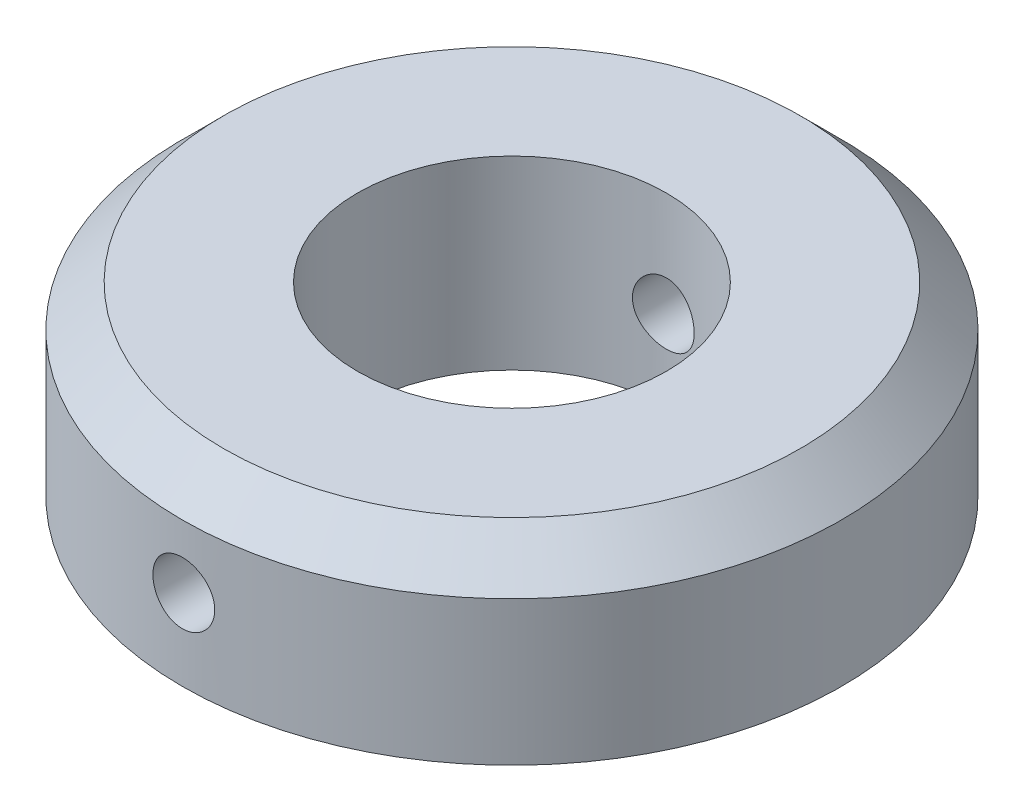
ISO-10303-21;
HEADER;
FILE_DESCRIPTION(('STEP AP214'),'2;1');
FILE_NAME('part.step','',(''),(''),'','','');
FILE_SCHEMA(('AUTOMOTIVE_DESIGN { 1 0 10303 214 1 1 1 1 }'));
ENDSEC;
DATA;
#1=APPLICATION_CONTEXT('core data for automotive mechanical design processes');
#2=APPLICATION_PROTOCOL_DEFINITION('international standard','automotive_design',2000,#1);
#3=PRODUCT_CONTEXT('',#1,'mechanical');
#4=PRODUCT('Part','Part','',(#3));
#5=PRODUCT_RELATED_PRODUCT_CATEGORY('part','',(#4));
#6=PRODUCT_DEFINITION_FORMATION('','',#4);
#7=PRODUCT_DEFINITION_CONTEXT('part definition',#1,'design');
#8=PRODUCT_DEFINITION('design','',#6,#7);
#9=PRODUCT_DEFINITION_SHAPE('','',#8);
#10=(LENGTH_UNIT() NAMED_UNIT(*) SI_UNIT(.MILLI.,.METRE.));
#11=(NAMED_UNIT(*) PLANE_ANGLE_UNIT() SI_UNIT($,.RADIAN.));
#12=(NAMED_UNIT(*) SI_UNIT($,.STERADIAN.) SOLID_ANGLE_UNIT());
#13=UNCERTAINTY_MEASURE_WITH_UNIT(LENGTH_MEASURE(1.E-05),#10,'distance_accuracy_value','');
#14=(GEOMETRIC_REPRESENTATION_CONTEXT(3) GLOBAL_UNCERTAINTY_ASSIGNED_CONTEXT((#13)) GLOBAL_UNIT_ASSIGNED_CONTEXT((#10,
#11,#12)) REPRESENTATION_CONTEXT('',''));
#15=CARTESIAN_POINT('',(0.,0.,0.));
#16=DIRECTION('',(0.,0.,1.));
#17=DIRECTION('',(1.,0.,0.));
#18=AXIS2_PLACEMENT_3D('',#15,#16,#17);
#19=CARTESIAN_POINT('',(0.,9.,0.));
#20=DIRECTION('',(0.,1.,0.));
#21=DIRECTION('',(0.,0.,1.));
#22=AXIS2_PLACEMENT_3D('',#19,#20,#21);
#23=PLANE('',#22);
#24=CARTESIAN_POINT('',(0.,9.,0.));
#25=DIRECTION('',(0.,1.,0.));
#26=DIRECTION('',(0.,0.,1.));
#27=AXIS2_PLACEMENT_3D('',#24,#25,#26);
#28=CIRCLE('',#27,14.);
#29=CARTESIAN_POINT('',(0.,9.,14.));
#30=VERTEX_POINT('',#29);
#31=EDGE_CURVE('E52',#30,#30,#28,.T.);
#32=ORIENTED_EDGE('',*,*,#31,.T.);
#33=EDGE_LOOP('',(#32));
#34=FACE_BOUND('',#33,.T.);
#35=CARTESIAN_POINT('',(0.,9.,0.));
#36=DIRECTION('',(0.,1.,0.));
#37=DIRECTION('',(0.,0.,1.));
#38=AXIS2_PLACEMENT_3D('',#35,#36,#37);
#39=CIRCLE('',#38,7.5);
#40=CARTESIAN_POINT('',(0.,9.,7.5));
#41=VERTEX_POINT('',#40);
#42=EDGE_CURVE('E110',#41,#41,#39,.T.);
#43=ORIENTED_EDGE('',*,*,#42,.F.);
#44=EDGE_LOOP('',(#43));
#45=FACE_BOUND('',#44,.T.);
#46=ADVANCED_FACE('F39',(#34,#45),#23,.T.);
#47=CARTESIAN_POINT('',(0.,0.,0.));
#48=DIRECTION('',(0.,1.,0.));
#49=DIRECTION('',(0.,0.,1.));
#50=AXIS2_PLACEMENT_3D('',#47,#48,#49);
#51=PLANE('',#50);
#52=CARTESIAN_POINT('',(0.,0.,0.));
#53=DIRECTION('',(0.,1.,0.));
#54=DIRECTION('',(0.,0.,1.));
#55=AXIS2_PLACEMENT_3D('',#52,#53,#54);
#56=CIRCLE('',#55,16.);
#57=CARTESIAN_POINT('',(0.,0.,16.));
#58=VERTEX_POINT('',#57);
#59=EDGE_CURVE('E59',#58,#58,#56,.T.);
#60=ORIENTED_EDGE('',*,*,#59,.F.);
#61=EDGE_LOOP('',(#60));
#62=FACE_BOUND('',#61,.T.);
#63=CARTESIAN_POINT('',(0.,0.,0.));
#64=DIRECTION('',(0.,1.,0.));
#65=DIRECTION('',(0.,0.,1.));
#66=AXIS2_PLACEMENT_3D('',#63,#64,#65);
#67=CIRCLE('',#66,7.5);
#68=CARTESIAN_POINT('',(0.,0.,7.5));
#69=VERTEX_POINT('',#68);
#70=EDGE_CURVE('E108',#69,#69,#67,.T.);
#71=ORIENTED_EDGE('',*,*,#70,.T.);
#72=EDGE_LOOP('',(#71));
#73=FACE_BOUND('',#72,.T.);
#74=ADVANCED_FACE('F91',(#62,#73),#51,.F.);
#75=CARTESIAN_POINT('',(0.,9.,0.));
#76=DIRECTION('',(0.,-1.,0.));
#77=DIRECTION('',(0.,0.,-1.));
#78=AXIS2_PLACEMENT_3D('',#75,#76,#77);
#79=CYLINDRICAL_SURFACE('',#78,16.);
#80=CARTESIAN_POINT('',(0.,5.43034536282499,-16.));
#81=CARTESIAN_POINT('',(-0.0840576996574437,5.43034170985044,-15.9999990874377));
#82=CARTESIAN_POINT('',(-0.168171627589379,5.423255885696,-15.9993305431474));
#83=CARTESIAN_POINT('',(-0.334069380755584,5.39509506295832,-15.9967278705616));
#84=CARTESIAN_POINT('',(-0.41585050405935,5.37400447917629,-15.9947923323258));
#85=CARTESIAN_POINT('',(-0.574656127608676,5.31845188267265,-15.9898742536092));
#86=CARTESIAN_POINT('',(-0.65168339804474,5.28399774416038,-15.9868923297887));
#87=CARTESIAN_POINT('',(-0.798844080486045,5.20271088579991,-15.9802152971296));
#88=CARTESIAN_POINT('',(-0.868978900331676,5.15588070110172,-15.9765203343939));
#89=CARTESIAN_POINT('',(-1.00060451358299,5.05101076457032,-15.9688182603974));
#90=CARTESIAN_POINT('',(-1.06207030524923,4.99293969202882,-15.9648102960756));
#91=CARTESIAN_POINT('',(-1.17439832001845,4.86730300549484,-15.9569410358395));
#92=CARTESIAN_POINT('',(-1.22526006263066,4.79973696149825,-15.9530797465779));
#93=CARTESIAN_POINT('',(-1.31502335742932,4.6568736146017,-15.9459321531903));
#94=CARTESIAN_POINT('',(-1.3539025185592,4.58156218431094,-15.9426469303983));
#95=CARTESIAN_POINT('',(-1.41845402355083,4.42544403169777,-15.9370337331836));
#96=CARTESIAN_POINT('',(-1.44412665669788,4.34463742978944,-15.9347057377932));
#97=CARTESIAN_POINT('',(-1.48146280171703,4.18007617451122,-15.9312781055131));
#98=CARTESIAN_POINT('',(-1.4931675262139,4.09633094808939,-15.9301748556596));
#99=CARTESIAN_POINT('',(-1.50236296529023,3.92805789753474,-15.9293103424401));
#100=CARTESIAN_POINT('',(-1.49985401107328,3.84353009168322,-15.9295490478042));
#101=CARTESIAN_POINT('',(-1.48072731632193,3.67637474710345,-15.9313381803757));
#102=CARTESIAN_POINT('',(-1.46415449112824,3.59374201798684,-15.9328844316596));
#103=CARTESIAN_POINT('',(-1.41744034122964,3.43243614206901,-15.9371079001961));
#104=CARTESIAN_POINT('',(-1.3872988532664,3.35376304292278,-15.9397851310565));
#105=CARTESIAN_POINT('',(-1.3142531244971,3.20246728495301,-15.9459737103685));
#106=CARTESIAN_POINT('',(-1.27132886758545,3.12985434553073,-15.9494863652322));
#107=CARTESIAN_POINT('',(-1.17395046357292,2.9928464513137,-15.9569488633928));
#108=CARTESIAN_POINT('',(-1.11949602014408,2.92845170779631,-15.9608987179246));
#109=CARTESIAN_POINT('',(-1.0003517239972,2.80944707192839,-15.9688091656293));
#110=CARTESIAN_POINT('',(-0.935623065481643,2.7548760222016,-15.9727697411833));
#111=CARTESIAN_POINT('',(-0.797902747560453,2.65736861347273,-15.980240887844));
#112=CARTESIAN_POINT('',(-0.724911080506018,2.61443226524064,-15.9837514585342));
#113=CARTESIAN_POINT('',(-0.572710457840157,2.54141496340302,-15.9899280035071));
#114=CARTESIAN_POINT('',(-0.493500599071182,2.51133588134771,-15.9925938548147));
#115=CARTESIAN_POINT('',(-0.331124322273424,2.46491490921607,-15.9967792828423));
#116=CARTESIAN_POINT('',(-0.247958008264099,2.44857265819436,-15.9982988896806));
#117=CARTESIAN_POINT('',(-0.0803661051891792,2.43013829263682,-16.0000167439267));
#118=CARTESIAN_POINT('',(0.00405353705355389,2.42799255769071,-16.0002199632847));
#119=CARTESIAN_POINT('',(0.17205127843741,2.43787144609971,-15.9992954563897));
#120=CARTESIAN_POINT('',(0.25562938753764,2.44989590155872,-15.9981677459063));
#121=CARTESIAN_POINT('',(0.419417565662278,2.48772937270583,-15.9947113308173));
#122=CARTESIAN_POINT('',(0.499633460781156,2.51351338202034,-15.9923848051808));
#123=CARTESIAN_POINT('',(0.654601026064808,2.57810841177009,-15.9867919001555));
#124=CARTESIAN_POINT('',(0.729352587838971,2.61691969052914,-15.9835255021299));
#125=CARTESIAN_POINT('',(0.871512627170616,2.70660122899258,-15.9764061412804));
#126=CARTESIAN_POINT('',(0.938898720136997,2.75750683429548,-15.9725514712721));
#127=CARTESIAN_POINT('',(1.06418863953514,2.86988117350934,-15.9646938863657));
#128=CARTESIAN_POINT('',(1.12209225711382,2.93135014001898,-15.9606909682048));
#129=CARTESIAN_POINT('',(1.22695884240091,3.06333978161952,-15.9529731744665));
#130=CARTESIAN_POINT('',(1.27388669789138,3.13388841685224,-15.9492592480101));
#131=CARTESIAN_POINT('',(1.35522852111172,3.28189637233934,-15.9425540145368));
#132=CARTESIAN_POINT('',(1.38964264189423,3.35935560805731,-15.9395626986821));
#133=CARTESIAN_POINT('',(1.44492091464444,3.51886401781301,-15.9346470864828));
#134=CARTESIAN_POINT('',(1.46580619653949,3.60090581582139,-15.9327211269093));
#135=CARTESIAN_POINT('',(1.49350258954047,3.76735064147414,-15.9301489811257));
#136=CARTESIAN_POINT('',(1.50031405119065,3.8517536102545,-15.9295027630406));
#137=CARTESIAN_POINT('',(1.49966491440228,4.02017592399092,-15.929563861851));
#138=CARTESIAN_POINT('',(1.49225947642594,4.1041954889146,-15.930265947437));
#139=CARTESIAN_POINT('',(1.46350215815381,4.26979160292843,-15.9329334080922));
#140=CARTESIAN_POINT('',(1.44215025977346,4.35136814885054,-15.9348987847997));
#141=CARTESIAN_POINT('',(1.38612086380733,4.50976370527025,-15.9398699587172));
#142=CARTESIAN_POINT('',(1.35144474478351,4.5865832069908,-15.9428756482903));
#143=CARTESIAN_POINT('',(1.26975707915473,4.73331997686405,-15.9495889947787));
#144=CARTESIAN_POINT('',(1.22274565072801,4.80323731113401,-15.9532966449687));
#145=CARTESIAN_POINT('',(1.1175144922873,4.93446768251109,-15.9610133498176));
#146=CARTESIAN_POINT('',(1.05925372920377,4.99574775354154,-15.9650234741094));
#147=CARTESIAN_POINT('',(0.933256833294973,5.10768719699359,-15.97288349636));
#148=CARTESIAN_POINT('',(0.865518425328446,5.15834401194823,-15.9767333555577));
#149=CARTESIAN_POINT('',(0.722325032343342,5.24768622001424,-15.9838478838907));
#150=CARTESIAN_POINT('',(0.646852995234792,5.28634436712216,-15.9871112141985));
#151=CARTESIAN_POINT('',(0.490507906890444,5.35038854209055,-15.9926700583075));
#152=CARTESIAN_POINT('',(0.409641110987895,5.37578965014847,-15.9949666711945));
#153=CARTESIAN_POINT('',(0.273590626043441,5.40621111478394,-15.997751278192));
#154=CARTESIAN_POINT('',(0.219278798513779,5.41524922609769,-15.9985906537126));
#155=CARTESIAN_POINT('',(0.109986004796567,5.42731753475249,-15.9997153122197));
#156=CARTESIAN_POINT('',(0.0550050409638892,5.43034775323081,-16.0000005971556));
#157=CARTESIAN_POINT('',(0.,5.43034536282499,-16.));
#158=B_SPLINE_CURVE_WITH_KNOTS('',3,(#80,#81,#82,#83,#84,#85,#86,#87,#88,#89,#90,#91,#92,#93,
#94,#95,#96,#97,#98,#99,#100,#101,#102,#103,#104,#105,#106,#107,#108,#109,#110,#111,#112,#113,
#114,#115,#116,#117,#118,#119,#120,#121,#122,#123,#124,#125,#126,#127,#128,#129,#130,#131,#132,
#133,#134,#135,#136,#137,#138,#139,#140,#141,#142,#143,#144,#145,#146,#147,#148,#149,#150,#151,
#152,#153,#154,#155,#156,#157),.UNSPECIFIED.,.T.,.F.,(4,2,2,2,2,2,2,2,2,2,2,2,2,2,2,2,2,2,2,2,2,
2,2,2,2,2,2,2,2,2,2,2,2,2,2,2,2,2,4),(0.,0.251972252870636,0.504225384091021,0.756330105411321,
1.00838322474624,1.26114902549997,1.51392627709208,1.7671730523228,2.02041428001784,
2.27290645171288,2.52539273992279,2.77707569221288,3.02876167283653,3.28084385105098,
3.53293250861135,3.78599701442565,4.03906175449559,4.29216331905139,4.54525823296866,
4.79739665595728,5.04953209150326,5.30121085328536,5.55289460601788,5.80532315252837,
6.05775725807137,6.31098819719604,6.56421603900671,6.81704741885484,7.06987250121943,
7.32171862414045,7.57356507363443,7.82538547338789,8.07720346066821,8.32995794997956,
8.58277321830877,8.8361584370252,9.08925479233284,9.25413906717824,9.41902276191882),.UNSPECIFIED.);
#159=CARTESIAN_POINT('',(0.,5.43034536282499,-16.));
#160=VERTEX_POINT('',#159);
#161=EDGE_CURVE('E85',#160,#160,#158,.T.);
#162=ORIENTED_EDGE('',*,*,#161,.T.);
#163=EDGE_LOOP('',(#162));
#164=FACE_BOUND('',#163,.T.);
#165=CARTESIAN_POINT('',(1.5,3.93034536282499,15.929532322074));
#166=CARTESIAN_POINT('',(1.49999634620447,3.84628857842711,15.9295332496796));
#167=CARTESIAN_POINT('',(1.49291067114191,3.76217556284008,15.9302048142922));
#168=CARTESIAN_POINT('',(1.46475049444749,3.59627970529378,15.9328182764505));
#169=CARTESIAN_POINT('',(1.44366040446064,3.51449956598149,15.9347615895481));
#170=CARTESIAN_POINT('',(1.38810925248868,3.3556960230131,15.9396965331442));
#171=CARTESIAN_POINT('',(1.35365608820284,3.27866984083425,15.9426875443425));
#172=CARTESIAN_POINT('',(1.27237152401549,3.13151098150667,15.9493801055301));
#173=CARTESIAN_POINT('',(1.22554265686883,3.06137689787688,15.9530815100911));
#174=CARTESIAN_POINT('',(1.12067405070444,2.92975045195916,15.9607911339043));
#175=CARTESIAN_POINT('',(1.062602696675,2.86828332491989,15.9648001986727));
#176=CARTESIAN_POINT('',(0.936964886657167,2.75595273324473,15.9726657227971));
#177=CARTESIAN_POINT('',(0.869398004306441,2.70508974500413,15.9765221752908));
#178=CARTESIAN_POINT('',(0.726533924195945,2.6153251486955,15.9836561919841));
#179=CARTESIAN_POINT('',(0.651222743202337,2.57644570262144,15.9869326789076));
#180=CARTESIAN_POINT('',(0.495105132470078,2.5118936020372,15.9925284235434));
#181=CARTESIAN_POINT('',(0.414298821735456,2.48622066162639,15.9948477019775));
#182=CARTESIAN_POINT('',(0.249738452457438,2.44888387300111,15.9982617839516));
#183=CARTESIAN_POINT('',(0.165993826496405,2.43717878581782,15.9993601913537));
#184=CARTESIAN_POINT('',(-0.00227804877261734,2.42798241333139,16.0002210112843));
#185=CARTESIAN_POINT('',(-0.0868052800149707,2.43049080073753,15.9999834545757));
#186=CARTESIAN_POINT('',(-0.253963127789742,2.44961659939017,15.9982020712559));
#187=CARTESIAN_POINT('',(-0.336598868002988,2.46618966582899,15.9966623503171));
#188=CARTESIAN_POINT('',(-0.497910641604227,2.51290534244825,15.9924544533603));
#189=CARTESIAN_POINT('',(-0.57658662892854,2.54304811044404,15.9897862642183));
#190=CARTESIAN_POINT('',(-0.727885882948087,2.61609648693961,15.9836144229149));
#191=CARTESIAN_POINT('',(-0.80049957541682,2.65902181244727,15.9801094817377));
#192=CARTESIAN_POINT('',(-0.937508522273802,2.75640249573777,15.9726576575237));
#193=CARTESIAN_POINT('',(-1.00190356497603,2.81085815040885,15.9687107631086));
#194=CARTESIAN_POINT('',(-1.12090682782472,2.93000330405911,15.9608002909644));
#195=CARTESIAN_POINT('',(-1.17547645005228,2.99473136195687,15.9568367074598));
#196=CARTESIAN_POINT('',(-1.27298126503045,3.13244997016446,15.9493547735685));
#197=CARTESIAN_POINT('',(-1.31591644407059,3.205440530211,15.9458364237066));
#198=CARTESIAN_POINT('',(-1.38893290545864,3.35764085650933,15.9396428732834));
#199=CARTESIAN_POINT('',(-1.41901195456847,3.43685170045994,15.9369678192323));
#200=CARTESIAN_POINT('',(-1.46543255875734,3.59923011815107,15.9327667240735));
#201=CARTESIAN_POINT('',(-1.48177448073806,3.68239758615236,15.9312406522781));
#202=CARTESIAN_POINT('',(-1.50020760574519,3.8499900204488,15.9295155036003));
#203=CARTESIAN_POINT('',(-1.50235273858312,3.93440900556563,15.9293114049579));
#204=CARTESIAN_POINT('',(-1.49247288052307,4.10240528792348,15.9302400596196));
#205=CARTESIAN_POINT('',(-1.48044805752832,4.18598259512589,15.9313727970831));
#206=CARTESIAN_POINT('',(-1.4426146852516,4.34976681280554,15.9348429214202));
#207=CARTESIAN_POINT('',(-1.41683150437604,4.42997963424203,15.9371780909077));
#208=CARTESIAN_POINT('',(-1.35223916126094,4.58494141882254,15.9427881521344));
#209=CARTESIAN_POINT('',(-1.31342973581779,4.65969027152639,15.9460630628614));
#210=CARTESIAN_POINT('',(-1.22375092063466,4.80184847311821,15.9531957731813));
#211=CARTESIAN_POINT('',(-1.17284571434593,4.86923514001278,15.957055291297));
#212=CARTESIAN_POINT('',(-1.06047184016521,4.99452640333808,15.9649166513233));
#213=CARTESIAN_POINT('',(-0.999002942454627,5.05243079342343,15.9689184963289));
#214=CARTESIAN_POINT('',(-0.86701296191927,5.15729903648996,15.9766286837569));
#215=CARTESIAN_POINT('',(-0.796463907072859,5.20422776406268,15.9803360594524));
#216=CARTESIAN_POINT('',(-0.648454880913737,5.28557111762231,15.9870255723539));
#217=CARTESIAN_POINT('',(-0.570994994266095,5.31998589689222,15.990007718443));
#218=CARTESIAN_POINT('',(-0.411487004753122,5.37526460763542,15.994906368584));
#219=CARTESIAN_POINT('',(-0.329446377285753,5.39614995432134,15.9968245560391));
#220=CARTESIAN_POINT('',(-0.163004019397259,5.42384687358065,15.9993860415818));
#221=CARTESIAN_POINT('',(-0.0786023467886059,5.43065879045037,16.0000293708579));
#222=CARTESIAN_POINT('',(0.0898207574367405,5.43001097679376,15.9999686642494));
#223=CARTESIAN_POINT('',(0.173842406331053,5.42260585826315,15.9992697841995));
#224=CARTESIAN_POINT('',(0.339442767773685,5.39384844555826,15.9966133623922));
#225=CARTESIAN_POINT('',(0.421021477800316,5.3724961369877,15.9946558193357));
#226=CARTESIAN_POINT('',(0.579421354861223,5.31646510942097,15.9897015157353));
#227=CARTESIAN_POINT('',(0.656243006946604,5.28178775171359,15.9867048613504));
#228=CARTESIAN_POINT('',(0.802983560308621,5.2000969433736,15.9800068530039));
#229=CARTESIAN_POINT('',(0.872902529034253,5.15308361329734,15.9763055059292));
#230=CARTESIAN_POINT('',(1.00413279287414,5.04785036840958,15.9685960985018));
#231=CARTESIAN_POINT('',(1.06541146913202,4.98958985510322,15.9645869596995));
#232=CARTESIAN_POINT('',(1.17734821522204,4.86359403193095,15.9567229915417));
#233=CARTESIAN_POINT('',(1.22800372394001,4.79585644380676,15.9528681995781));
#234=CARTESIAN_POINT('',(1.31734453209866,4.65266371370511,15.9457399565168));
#235=CARTESIAN_POINT('',(1.35600234935765,4.57719137229714,15.9424678473209));
#236=CARTESIAN_POINT('',(1.42004582325491,4.42084563745317,15.9368915656254));
#237=CARTESIAN_POINT('',(1.44544656465812,4.33997850130468,15.934586293585));
#238=CARTESIAN_POINT('',(1.4758669922284,4.20392899803419,15.9317906324285));
#239=CARTESIAN_POINT('',(1.48490463682216,4.14961856576008,15.9309477263712));
#240=CARTESIAN_POINT('',(1.49697232542926,4.04032856756397,15.9298182686926));
#241=CARTESIAN_POINT('',(1.50000239090824,3.98534900403356,15.9295317150833));
#242=CARTESIAN_POINT('',(1.5,3.93034536282499,15.929532322074));
#243=B_SPLINE_CURVE_WITH_KNOTS('',3,(#165,#166,#167,#168,#169,#170,#171,#172,#173,#174,#175,
#176,#177,#178,#179,#180,#181,#182,#183,#184,#185,#186,#187,#188,#189,#190,#191,#192,#193,#194,
#195,#196,#197,#198,#199,#200,#201,#202,#203,#204,#205,#206,#207,#208,#209,#210,#211,#212,#213,
#214,#215,#216,#217,#218,#219,#220,#221,#222,#223,#224,#225,#226,#227,#228,#229,#230,#231,#232,
#233,#234,#235,#236,#237,#238,#239,#240,#241,#242),.UNSPECIFIED.,.T.,.F.,(4,2,2,2,2,2,2,2,2,2,2,
2,2,2,2,2,2,2,2,2,2,2,2,2,2,2,2,2,2,2,2,2,2,2,2,2,2,2,4),(0.,0.251969503716216,
0.504219946620975,0.756321533813657,1.00837156694704,1.26114096513842,1.51392171665298,
1.76716718634083,2.02040717342109,2.27289762511177,2.52538226278092,2.77707378155992,
3.02876822758193,3.28085293951864,3.53294414303803,3.78600501892853,4.03906619303429,
4.29217130854314,4.54526966371245,4.79740601119813,5.04953937108953,5.30120943212744,
5.55288457862632,5.80531445139059,6.0577498165933,6.31098232163707,6.56421172473816,
6.81703931507447,7.0698607200925,7.32171290329082,7.573565346451,7.82539206716958,
8.07721632694076,8.32996718257734,8.58277890344214,8.83616551779352,9.0892631802755,
9.25414326458754,9.41902275976672),.UNSPECIFIED.);
#244=CARTESIAN_POINT('',(1.5,3.93034536282499,15.929532322074));
#245=VERTEX_POINT('',#244);
#246=EDGE_CURVE('E80',#245,#245,#243,.T.);
#247=ORIENTED_EDGE('',*,*,#246,.T.);
#248=EDGE_LOOP('',(#247));
#249=FACE_BOUND('',#248,.T.);
#250=CARTESIAN_POINT('',(0.,6.99999999999999,0.));
#251=DIRECTION('',(0.,1.,0.));
#252=DIRECTION('',(0.,0.,1.));
#253=AXIS2_PLACEMENT_3D('',#250,#251,#252);
#254=CIRCLE('',#253,16.);
#255=CARTESIAN_POINT('',(0.,6.99999999999999,16.));
#256=VERTEX_POINT('',#255);
#257=EDGE_CURVE('E10',#256,#256,#254,.F.);
#258=ORIENTED_EDGE('',*,*,#257,.T.);
#259=EDGE_LOOP('',(#258));
#260=FACE_BOUND('',#259,.T.);
#261=ORIENTED_EDGE('',*,*,#59,.T.);
#262=EDGE_LOOP('',(#261));
#263=FACE_BOUND('',#262,.T.);
#264=ADVANCED_FACE('F90',(#164,#249,#260,#263),#79,.T.);
#265=CARTESIAN_POINT('',(0.,9.,0.));
#266=DIRECTION('',(0.,-1.,0.));
#267=DIRECTION('',(0.,0.,-1.));
#268=AXIS2_PLACEMENT_3D('',#265,#266,#267);
#269=CYLINDRICAL_SURFACE('',#268,7.5);
#270=CARTESIAN_POINT('',(0.,5.43034536282499,-7.5));
#271=CARTESIAN_POINT('',(-0.0833653601889498,5.43034229607747,-7.49999846371307));
#272=CARTESIAN_POINT('',(-0.166769490302284,5.42337209837352,-7.49859577767346));
#273=CARTESIAN_POINT('',(-0.331220261533529,5.39569761265212,-7.49313548434847));
#274=CARTESIAN_POINT('',(-0.412264976312034,5.37498241362273,-7.48907576790279));
#275=CARTESIAN_POINT('',(-0.56959545789497,5.32048345239381,-7.4787547391743));
#276=CARTESIAN_POINT('',(-0.645885701899702,5.28671220755796,-7.47249553615077));
#277=CARTESIAN_POINT('',(-0.791711983296339,5.20709699155805,-7.45845597052971));
#278=CARTESIAN_POINT('',(-0.861248422613718,5.16125373941418,-7.4506756985356));
#279=CARTESIAN_POINT('',(-0.992540215972298,5.05813762138784,-7.43433247994955));
#280=CARTESIAN_POINT('',(-1.05419092673779,5.00073282973819,-7.42576118256521));
#281=CARTESIAN_POINT('',(-1.16705513491204,4.87640673823744,-7.40886270678882));
#282=CARTESIAN_POINT('',(-1.21826781715564,4.80948469582231,-7.40053554750636));
#283=CARTESIAN_POINT('',(-1.30924763002143,4.66727107330718,-7.38498662718923));
#284=CARTESIAN_POINT('',(-1.3489064082988,4.59190889713045,-7.37777561047419));
#285=CARTESIAN_POINT('',(-1.41495849987046,4.43542263431887,-7.36539402087627));
#286=CARTESIAN_POINT('',(-1.44135312365586,4.35429911780547,-7.36022324642942));
#287=CARTESIAN_POINT('',(-1.47978794982724,4.18971881696311,-7.35259207878307));
#288=CARTESIAN_POINT('',(-1.49201174693817,4.10630654661165,-7.35009705160781));
#289=CARTESIAN_POINT('',(-1.50232819158918,3.93858063077848,-7.34799562590941));
#290=CARTESIAN_POINT('',(-1.50042228407025,3.85426707834477,-7.34838893201761));
#291=CARTESIAN_POINT('',(-1.48268185965273,3.68847518079349,-7.35198826722277));
#292=CARTESIAN_POINT('',(-1.46705781036586,3.60697325438402,-7.35515179288145));
#293=CARTESIAN_POINT('',(-1.42265682693458,3.44777124783049,-7.36386819240002));
#294=CARTESIAN_POINT('',(-1.39387926465102,3.37007134944648,-7.36942118036668));
#295=CARTESIAN_POINT('',(-1.32378717551208,3.22007247026959,-7.38233427750612));
#296=CARTESIAN_POINT('',(-1.28238922684817,3.14781354347123,-7.38970634720557));
#297=CARTESIAN_POINT('',(-1.18829036185902,3.01118908786577,-7.40541928159593));
#298=CARTESIAN_POINT('',(-1.13558814653524,2.94682446754825,-7.41376025757549));
#299=CARTESIAN_POINT('',(-1.01924990184088,2.82660125913959,-7.43065531862193));
#300=CARTESIAN_POINT('',(-0.955434241818667,2.77091651103629,-7.43921053816357));
#301=CARTESIAN_POINT('',(-0.819277536093014,2.67101459337315,-7.45543273071613));
#302=CARTESIAN_POINT('',(-0.746936381069083,2.62679757088462,-7.4630996923346));
#303=CARTESIAN_POINT('',(-0.595589080318381,2.55105409898603,-7.47670035241331));
#304=CARTESIAN_POINT('',(-0.51657272937795,2.51954752235818,-7.48263133272408));
#305=CARTESIAN_POINT('',(-0.354223464672997,2.47030465176714,-7.49207113481787));
#306=CARTESIAN_POINT('',(-0.270891075108674,2.45256668971455,-7.49558025000797));
#307=CARTESIAN_POINT('',(-0.103769108440726,2.43161068213357,-7.49974007800302));
#308=CARTESIAN_POINT('',(-0.0200104924883643,2.42815473351459,-7.50043761978705));
#309=CARTESIAN_POINT('',(0.146887401289071,2.43522015123826,-7.49902577895154));
#310=CARTESIAN_POINT('',(0.23002671366569,2.44574073185388,-7.49691655412169));
#311=CARTESIAN_POINT('',(0.392558489919811,2.48026292314092,-7.49015748012026));
#312=CARTESIAN_POINT('',(0.471977922509855,2.50414246557184,-7.4855306460631));
#313=CARTESIAN_POINT('',(0.625685441249501,2.5645713368087,-7.47425328091549));
#314=CARTESIAN_POINT('',(0.699973142456309,2.60112161484024,-7.4676025982134));
#315=CARTESIAN_POINT('',(0.842311760529326,2.68636909880196,-7.45289867299942));
#316=CARTESIAN_POINT('',(0.910275190128282,2.73520953438341,-7.44482925655578));
#317=CARTESIAN_POINT('',(1.03712702867881,2.84345914963591,-7.42822102244824));
#318=CARTESIAN_POINT('',(1.09601446339614,2.90286946242479,-7.41968215452582));
#319=CARTESIAN_POINT('',(1.20396088616126,3.03165539066168,-7.40293955335447));
#320=CARTESIAN_POINT('',(1.25285655367298,3.101168979157,-7.39474290349956));
#321=CARTESIAN_POINT('',(1.33827813007681,3.24756240486001,-7.37976287694291));
#322=CARTESIAN_POINT('',(1.37480453388435,3.32444194718532,-7.37297944370014));
#323=CARTESIAN_POINT('',(1.43422776237294,3.48299773204931,-7.36165110876574));
#324=CARTESIAN_POINT('',(1.45719524968658,3.56464662464047,-7.3570946230828));
#325=CARTESIAN_POINT('',(1.48906297744079,3.73074554306135,-7.35071155188038));
#326=CARTESIAN_POINT('',(1.49796505233767,3.81519520213901,-7.34888461036667));
#327=CARTESIAN_POINT('',(1.5013813663012,3.98285865964147,-7.34818724447069));
#328=CARTESIAN_POINT('',(1.49615368210634,4.0660670862155,-7.34926378783951));
#329=CARTESIAN_POINT('',(1.47202845615009,4.23039283768253,-7.35413360226921));
#330=CARTESIAN_POINT('',(1.45313102419395,4.3115101793672,-7.35792685150754));
#331=CARTESIAN_POINT('',(1.40231785274843,4.46918692968581,-7.36777896328738));
#332=CARTESIAN_POINT('',(1.37043376007602,4.54575690357861,-7.37383231528246));
#333=CARTESIAN_POINT('',(1.29458196690241,4.69250094392665,-7.38752572461255));
#334=CARTESIAN_POINT('',(1.25061325316232,4.7626744734127,-7.39516591498341));
#335=CARTESIAN_POINT('',(1.15095887217962,4.89591872105046,-7.41133440784838));
#336=CARTESIAN_POINT('',(1.09508683085277,4.95884851072638,-7.41987559364549));
#337=CARTESIAN_POINT('',(0.973596553519711,5.07452467111875,-7.43679122807932));
#338=CARTESIAN_POINT('',(0.907976080730002,5.1272686983009,-7.44516563794777));
#339=CARTESIAN_POINT('',(0.768026443632369,5.22159732874466,-7.46090748581957));
#340=CARTESIAN_POINT('',(0.693613326644751,5.26305936774503,-7.46826346828869));
#341=CARTESIAN_POINT('',(0.538749541411098,5.33282454671988,-7.481026876275));
#342=CARTESIAN_POINT('',(0.458304391294689,5.36113954712373,-7.48643605707924));
#343=CARTESIAN_POINT('',(0.314732233385669,5.39832328489207,-7.49364558893056));
#344=CARTESIAN_POINT('',(0.252422496020677,5.41031015338663,-7.49601454737677));
#345=CARTESIAN_POINT('',(0.1267492878151,5.42632223136254,-7.49919231209839));
#346=CARTESIAN_POINT('',(0.0633858506229285,5.43034769458964,-7.50000116809732));
#347=CARTESIAN_POINT('',(0.,5.43034536282499,-7.5));
#348=B_SPLINE_CURVE_WITH_KNOTS('',3,(#270,#271,#272,#273,#274,#275,#276,#277,#278,#279,#280,
#281,#282,#283,#284,#285,#286,#287,#288,#289,#290,#291,#292,#293,#294,#295,#296,#297,#298,#299,
#300,#301,#302,#303,#304,#305,#306,#307,#308,#309,#310,#311,#312,#313,#314,#315,#316,#317,#318,
#319,#320,#321,#322,#323,#324,#325,#326,#327,#328,#329,#330,#331,#332,#333,#334,#335,#336,#337,
#338,#339,#340,#341,#342,#343,#344,#345,#346,#347),.UNSPECIFIED.,.T.,.F.,(4,2,2,2,2,2,2,2,2,2,2,
2,2,2,2,2,2,2,2,2,2,2,2,2,2,2,2,2,2,2,2,2,2,2,2,2,2,2,4),(0.,0.249864195991888,
0.499926976036985,0.749750602875513,0.999559353346295,1.25239900516828,1.50525839512105,
1.76041792508884,2.01555224047796,2.26734277655381,2.51910756421838,2.76707590509417,
3.01505608880595,3.26471235305389,3.51439732124506,3.76857378737026,4.0227535130973,
4.27732912281036,4.53187388547054,4.78216103514398,5.03243411486801,5.28045680926085,
5.52849808824034,5.77957599050038,6.03068082518895,6.28560942868839,6.540527830852,
6.79410571549085,7.04765052495622,7.29659583851552,7.54553915238913,7.79387941879665,
8.042240513728,8.29482114358715,8.54745981799396,8.80274245013456,9.05779433276278,
9.24778162934841,9.43776287056494),.UNSPECIFIED.);
#349=CARTESIAN_POINT('',(0.,5.43034536282499,-7.5));
#350=VERTEX_POINT('',#349);
#351=EDGE_CURVE('E42',#350,#350,#348,.T.);
#352=ORIENTED_EDGE('',*,*,#351,.F.);
#353=EDGE_LOOP('',(#352));
#354=FACE_BOUND('',#353,.T.);
#355=CARTESIAN_POINT('',(1.5,3.93034536282499,7.34846922834953));
#356=CARTESIAN_POINT('',(1.49999691881235,3.84699879958923,7.34847088538349));
#357=CARTESIAN_POINT('',(1.49302975757707,3.76361342782524,7.34990262402618));
#358=CARTESIAN_POINT('',(1.46536842537441,3.59920160511003,7.35546646957746));
#359=CARTESIAN_POINT('',(1.44466327060578,3.51817709587095,7.35960073717297));
#360=CARTESIAN_POINT('',(1.39019367392958,3.36088940779374,7.37008310582665));
#361=CARTESIAN_POINT('',(1.35644222122892,3.28462158052613,7.37642900431582));
#362=CARTESIAN_POINT('',(1.27687366150577,3.13883309577954,7.39061699221019));
#363=CARTESIAN_POINT('',(1.23105722790173,3.06931206201813,7.398458998102));
#364=CARTESIAN_POINT('',(1.12796861348015,2.9380038570442,7.4148794954137));
#365=CARTESIAN_POINT('',(1.07055848386998,2.87632598099903,7.42346606755867));
#366=CARTESIAN_POINT('',(0.946210183531967,2.76340906245652,7.440337084539));
#367=CARTESIAN_POINT('',(0.879271345466977,2.7121707516992,7.44862150816248));
#368=CARTESIAN_POINT('',(0.737042033886384,2.6211633363823,7.46404194626342));
#369=CARTESIAN_POINT('',(0.661683851508316,2.58149809210003,7.47116732162326));
#370=CARTESIAN_POINT('',(0.505206225580908,2.51543295725279,7.48337605325447));
#371=CARTESIAN_POINT('',(0.42408732213083,2.4890318249735,7.48845960066179));
#372=CARTESIAN_POINT('',(0.259525159917742,2.45058457239555,7.49595481032628));
#373=CARTESIAN_POINT('',(0.176126608822222,2.43835389646848,7.4984007943219));
#374=CARTESIAN_POINT('',(0.00842785265630517,2.42801893506752,7.50046381775405));
#375=CARTESIAN_POINT('',(-0.075872264747764,2.42991328835626,7.50008112979138));
#376=CARTESIAN_POINT('',(-0.241713001115382,2.44763463314832,7.49655652302773));
#377=CARTESIAN_POINT('',(-0.323275821447704,2.46326282857676,7.49345397548757));
#378=CARTESIAN_POINT('',(-0.482597439870451,2.50769291151333,7.48488265739113));
#379=CARTESIAN_POINT('',(-0.560356085620693,2.5364953261128,7.47941379216059));
#380=CARTESIAN_POINT('',(-0.71042919480133,2.60664042304589,7.46665944029938));
#381=CARTESIAN_POINT('',(-0.782706261200849,2.64806098948232,7.45936272262835));
#382=CARTESIAN_POINT('',(-0.919357568789633,2.74220897867989,7.44375704210678));
#383=CARTESIAN_POINT('',(-0.983730899287501,2.79493770248076,7.43544796282833));
#384=CARTESIAN_POINT('',(-1.10392714658019,2.9112957959877,7.41856446546689));
#385=CARTESIAN_POINT('',(-1.15958147486045,2.97509914291937,7.40998794686274));
#386=CARTESIAN_POINT('',(-1.25942773976521,3.11122002650112,7.39367357398141));
#387=CARTESIAN_POINT('',(-1.30361945959163,3.18353772414978,7.38593573556822));
#388=CARTESIAN_POINT('',(-1.37934422220282,3.3348766105577,7.37217071209385));
#389=CARTESIAN_POINT('',(-1.41084997166656,3.41391181428448,7.36614722345324));
#390=CARTESIAN_POINT('',(-1.46008551244137,3.57630234841098,7.35654714481909));
#391=CARTESIAN_POINT('',(-1.47781709918496,3.65965711425362,7.35297023592642));
#392=CARTESIAN_POINT('',(-1.49874900905408,3.82679264982356,7.34873218901742));
#393=CARTESIAN_POINT('',(-1.50219278834687,3.9105417242905,7.34802220585731));
#394=CARTESIAN_POINT('',(-1.49510644246611,4.07741769762452,7.34946728533281));
#395=CARTESIAN_POINT('',(-1.48457710968366,4.16054463150329,7.35162218550582));
#396=CARTESIAN_POINT('',(-1.45005331211124,4.32299832326334,7.35850848742372));
#397=CARTESIAN_POINT('',(-1.42618893125895,4.40235387737864,7.36321498521745));
#398=CARTESIAN_POINT('',(-1.36581155296278,4.5559402813681,7.37465234027497));
#399=CARTESIAN_POINT('',(-1.32929751355977,4.63017070847857,7.38138336429404));
#400=CARTESIAN_POINT('',(-1.2441062133234,4.77246502775023,7.39622108943059));
#401=CARTESIAN_POINT('',(-1.19527661697413,4.84043593227623,7.40434457797355));
#402=CARTESIAN_POINT('',(-1.08704335831907,4.96730783082636,7.42100585739955));
#403=CARTESIAN_POINT('',(-1.02763860771681,5.02620789019887,7.42954369085727));
#404=CARTESIAN_POINT('',(-0.898848410246836,5.13418920160336,7.44623018803823));
#405=CARTESIAN_POINT('',(-0.829323748394444,5.18310584479999,7.45437086563026));
#406=CARTESIAN_POINT('',(-0.682901844952133,5.26856418507437,7.4692069144293));
#407=CARTESIAN_POINT('',(-0.60600491315026,5.30510640184216,7.47590234632816));
#408=CARTESIAN_POINT('',(-0.44745402123602,5.36453867044494,7.487059410916));
#409=CARTESIAN_POINT('',(-0.365830010217117,5.38750614016437,7.49153368713906));
#410=CARTESIAN_POINT('',(-0.199784182019869,5.41938223432076,7.4977985390649));
#411=CARTESIAN_POINT('',(-0.115362703066822,5.42829255203851,7.49958943799765));
#412=CARTESIAN_POINT('',(0.0523093408554345,5.43173583426932,7.50027810681181));
#413=CARTESIAN_POINT('',(0.135554718212253,5.42651628350931,7.49922567824026));
#414=CARTESIAN_POINT('',(0.299956546973461,5.40239443700327,7.49445065340477));
#415=CARTESIAN_POINT('',(0.381113024630536,5.38349231330288,7.49072809071528));
#416=CARTESIAN_POINT('',(0.538879124617644,5.33265187468752,7.481032475475));
#417=CARTESIAN_POINT('',(0.615498664860421,5.30074329562821,7.47506455871866));
#418=CARTESIAN_POINT('',(0.762331830278928,5.22482700082864,7.46152083185077));
#419=CARTESIAN_POINT('',(0.832544948651117,5.18081832896942,7.45394489468828));
#420=CARTESIAN_POINT('',(0.965795835159535,5.08111628223187,7.43786398736791));
#421=CARTESIAN_POINT('',(1.02869957417475,5.02524585824483,7.4293460013317));
#422=CARTESIAN_POINT('',(1.14432392663527,4.90377000268134,7.41241834355477));
#423=CARTESIAN_POINT('',(1.19704212480408,4.83816226862192,7.40400869794476));
#424=CARTESIAN_POINT('',(1.29133832918279,4.69822638777469,7.3881501412478));
#425=CARTESIAN_POINT('',(1.33279022195961,4.6238119210843,7.38071255446371));
#426=CARTESIAN_POINT('',(1.40253607393175,4.46894620287559,7.36777855777287));
#427=CARTESIAN_POINT('',(1.43084196896908,4.38850050477865,7.36228038807748));
#428=CARTESIAN_POINT('',(1.4680037097813,4.24495167966974,7.3549452169166));
#429=CARTESIAN_POINT('',(1.47998084778413,4.1826672335565,7.35253177367824));
#430=CARTESIAN_POINT('',(1.49598002694097,4.05704443099584,7.34929317692711));
#431=CARTESIAN_POINT('',(1.50000234234439,3.99370611095755,7.34846796865859));
#432=CARTESIAN_POINT('',(1.5,3.93034536282499,7.34846922834953));
#433=B_SPLINE_CURVE_WITH_KNOTS('',3,(#355,#356,#357,#358,#359,#360,#361,#362,#363,#364,#365,
#366,#367,#368,#369,#370,#371,#372,#373,#374,#375,#376,#377,#378,#379,#380,#381,#382,#383,#384,
#385,#386,#387,#388,#389,#390,#391,#392,#393,#394,#395,#396,#397,#398,#399,#400,#401,#402,#403,
#404,#405,#406,#407,#408,#409,#410,#411,#412,#413,#414,#415,#416,#417,#418,#419,#420,#421,#422,
#423,#424,#425,#426,#427,#428,#429,#430,#431,#432),.UNSPECIFIED.,.T.,.F.,(4,2,2,2,2,2,2,2,2,2,2,
2,2,2,2,2,2,2,2,2,2,2,2,2,2,2,2,2,2,2,2,2,2,2,2,2,2,2,4),(0.,0.249807695804142,
0.499815358926445,0.749574746910879,0.999320197289795,1.25223378822655,1.50516510053133,
1.76030100656175,2.0154130236984,2.26716373324621,2.51889018174372,2.76703184450306,
3.01518343610625,3.26489886333455,3.51464303655099,3.76874020143725,4.0228421718408,
4.27748794759165,4.53210052524037,4.7823563670689,5.03259801792632,5.28044012674978,
5.52830265531597,5.77939589661782,6.03051499305313,6.28548902600176,6.54045234945157,
6.79394720367975,7.04741152037442,7.29646526122029,7.54551587050135,7.79400025613178,
8.04250428202026,8.29501728038395,8.54759008334672,8.80288347868562,9.05794462633399,
9.24785705455344,9.43776293526322),.UNSPECIFIED.);
#434=CARTESIAN_POINT('',(1.5,3.93034536282499,7.34846922834953));
#435=VERTEX_POINT('',#434);
#436=EDGE_CURVE('E63',#435,#435,#433,.T.);
#437=ORIENTED_EDGE('',*,*,#436,.F.);
#438=EDGE_LOOP('',(#437));
#439=FACE_BOUND('',#438,.T.);
#440=ORIENTED_EDGE('',*,*,#42,.T.);
#441=EDGE_LOOP('',(#440));
#442=FACE_BOUND('',#441,.T.);
#443=ORIENTED_EDGE('',*,*,#70,.F.);
#444=EDGE_LOOP('',(#443));
#445=FACE_BOUND('',#444,.T.);
#446=ADVANCED_FACE('F68',(#354,#439,#442,#445),#269,.F.);
#447=CARTESIAN_POINT('',(0.,9.,0.));
#448=DIRECTION('',(0.,-1.,0.));
#449=DIRECTION('',(0.,0.,-1.));
#450=AXIS2_PLACEMENT_3D('',#447,#448,#449);
#451=CONICAL_SURFACE('',#450,14.,0.785398163397447);
#452=ORIENTED_EDGE('',*,*,#257,.F.);
#453=EDGE_LOOP('',(#452));
#454=FACE_BOUND('',#453,.T.);
#455=ORIENTED_EDGE('',*,*,#31,.F.);
#456=EDGE_LOOP('',(#455));
#457=FACE_BOUND('',#456,.T.);
#458=ADVANCED_FACE('F45',(#454,#457),#451,.T.);
#459=CARTESIAN_POINT('',(0.,3.93034536282499,-16.));
#460=DIRECTION('',(0.,0.,1.));
#461=DIRECTION('',(1.,0.,0.));
#462=AXIS2_PLACEMENT_3D('',#459,#460,#461);
#463=CYLINDRICAL_SURFACE('',#462,1.5);
#464=ORIENTED_EDGE('',*,*,#436,.T.);
#465=EDGE_LOOP('',(#464));
#466=FACE_BOUND('',#465,.T.);
#467=ORIENTED_EDGE('',*,*,#246,.F.);
#468=EDGE_LOOP('',(#467));
#469=FACE_BOUND('',#468,.T.);
#470=ADVANCED_FACE('F75',(#466,#469),#463,.F.);
#471=ORIENTED_EDGE('',*,*,#351,.T.);
#472=EDGE_LOOP('',(#471));
#473=FACE_BOUND('',#472,.T.);
#474=ORIENTED_EDGE('',*,*,#161,.F.);
#475=EDGE_LOOP('',(#474));
#476=FACE_BOUND('',#475,.T.);
#477=ADVANCED_FACE('F70',(#473,#476),#463,.F.);
#478=CLOSED_SHELL('',(#46,#74,#264,#446,#458,#470,#477));
#479=MANIFOLD_SOLID_BREP('B2',#478);
#480=ADVANCED_BREP_SHAPE_REPRESENTATION('',(#18,#479),#14);
#481=SHAPE_DEFINITION_REPRESENTATION(#9,#480);
ENDSEC;
END-ISO-10303-21;
